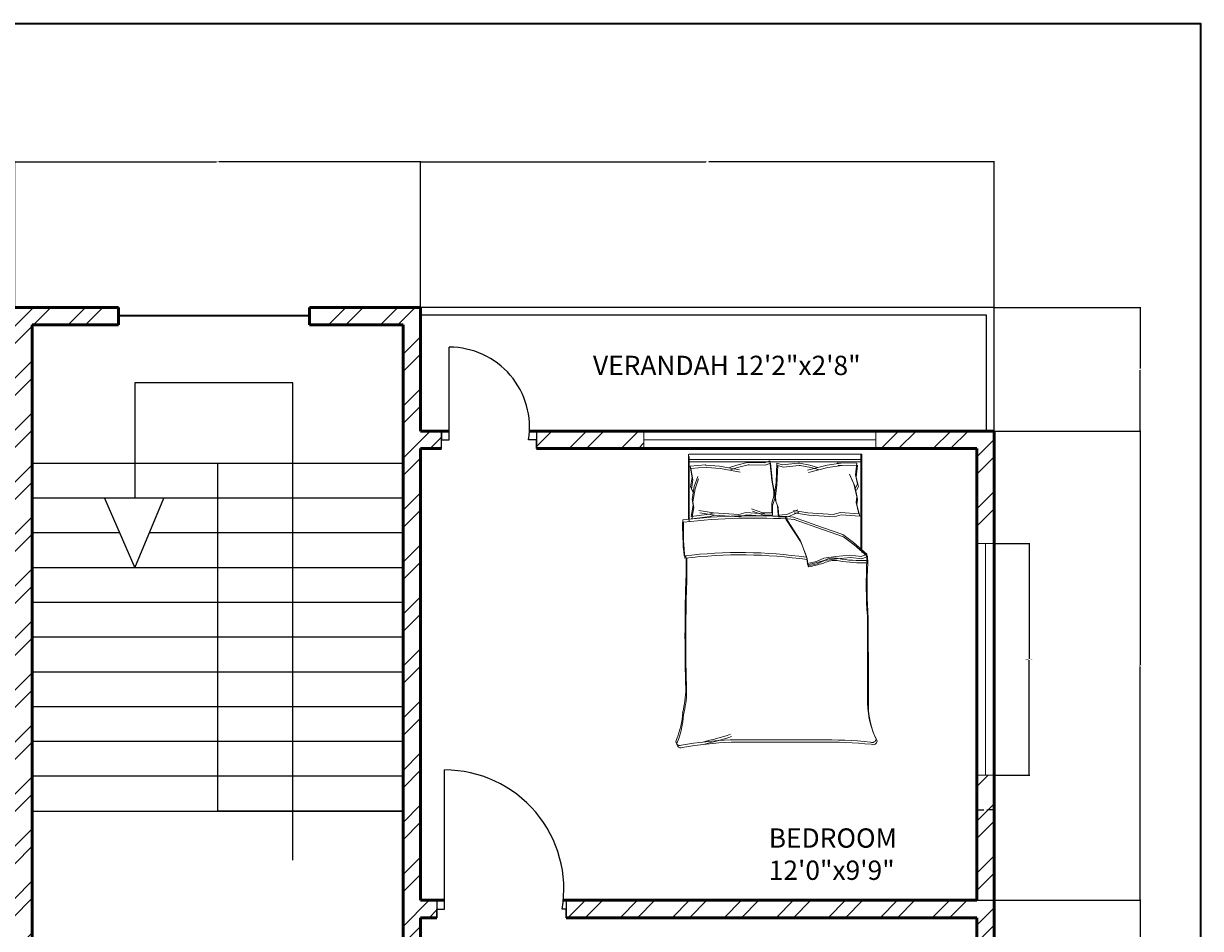
# Model space of a CAD drawing. Units: inches. Extents: x 2129 to 2642, y 1542 to 2414.
# Tile 9 of 9: x 2338 to 2642, y 2179 to 2414. Entities that reach past the tile are written whole.
import ezdxf

# ---------------------------------------------------------------- set-up
doc = ezdxf.new("R2010")
doc.units = ezdxf.units.IN
for name, color, linetype, lineweight in [('A-ANNO-DIMS', 2, 'Continuous', 18), ('A-ANNO-TTLB', 7, 'Continuous', 35), ('A-AREA-IDEN', 7, 'Continuous', 18), ('A-DOOR', 3, 'Continuous', 25), ('A-FLOR-RAIL', 80, 'Continuous', 25), ('A-FLOR-STRS', 11, 'Continuous', 25), ('A-FURN', 8, 'Continuous', 18), ('A-GLAZ', 4, 'Continuous', 18), ('A-WALL', 7, 'Continuous', 50), ('A-WALL-PATT', 252, 'Continuous', 13)]:
    doc.layers.add(name, color=color, linetype=linetype, lineweight=lineweight)
doc.styles.get("Standard").update_dxf_attribs({"font": 'arial.ttf'})
doc.dimstyles.get("Standard").update_dxf_attribs({"dimtxt": 0.18, "dimasz": 0.18, "dimexe": 0.18, "dimexo": 0.0625, "dimgap": 0.09, "dimtad": 0, "dimtih": 1, "dimtoh": 1, "dimdec": 4, "dimzin": 0, "dimdsep": 46, "dimtxsty": 'Standard', "dimcen": 0.09, "dimadec": 0, "dimazin": 0, "dimtfac": 1, "dimtdec": 4, "dimtofl": 0, "dimtmove": 0, "dimatfit": 3, "dimfxl": 1, "dimtolj": 1, "dimtzin": 0, "dimarcsym": 0})

# ---------------------------------------------------------------- blocks, each defined once
blk = doc.blocks.new('BED-DOUBLE')
for p, q in [((3.24, 59.14), (3.24, 76.05)), ((3.24, 74.61), (47.87, 74.61)), ((3.25, 59.14), (3.25, 76.05)), ((3.25, 74.61), (47.87, 74.61)), ((48.08, 76.05), (3.46, 76.05)), ((3.46, 58.54), (3.46, 75.45)), ((3.46, 58.54), (3.46, 75.45)), ((3.46, 74.02), (48.08, 74.02)), ((3.46, 74.02), (48.08, 74.02)), ((3.64, 72.93), (7.64, 73.24)), ((3.64, 72.93), (7.64, 73.24)), ((7.64, 73.24), (7.74, 73.22)), ((7.64, 73.24), (7.74, 73.22)), ((7.74, 73.22), (11.31, 72.95)), ((7.74, 73.22), (11.31, 72.95)), ((13.87, 72.55), (15.76, 73.22)), ((13.87, 72.55), (15.76, 73.22)), ((15.76, 73.22), (18.46, 73.9)), ((15.76, 73.22), (18.46, 73.9)), ((15.97, 72.62), (18.67, 73.3)), ((15.97, 72.62), (18.67, 73.3)), ((18.46, 73.9), (18.76, 73.9)), ((18.46, 73.9), (18.76, 73.9)), ((18.67, 73.3), (18.97, 73.3)), ((18.67, 73.3), (18.97, 73.3)), ((18.76, 73.9), (22.91, 73.76)), ((18.76, 73.9), (22.91, 73.76)), ((18.97, 73.3), (23.12, 73.16)), ((18.97, 73.3), (23.12, 73.16)), ((22.91, 73.76), (24.26, 74.3)), ((22.91, 73.76), (24.26, 74.3)), ((23.12, 73.16), (24.47, 73.7)), ((23.12, 73.16), (24.47, 73.7)), ((24.26, 74.3), (24.8, 69.31)), ((24.26, 74.3), (24.8, 69.31)), ((24.47, 73.7), (25.01, 68.71)), ((24.47, 73.7), (25.01, 68.71)), ((26.12, 73.72), (25.9, 68.7)), ((26.12, 73.72), (25.9, 68.7)), ((26.34, 73.12), (26.11, 68.1)), ((26.34, 73.12), (26.11, 68.1)), ((27.5, 73.27), (26.12, 73.72)), ((27.5, 73.27), (26.12, 73.72)), ((27.72, 72.67), (26.34, 73.12)), ((27.72, 72.67), (26.34, 73.12)), ((31.64, 73.66), (27.5, 73.27)), ((31.64, 73.66), (27.5, 73.27)), ((31.94, 73.68), (31.64, 73.66)), ((31.94, 73.68), (31.64, 73.66)), ((34.68, 73.17), (31.94, 73.68)), ((34.67, 73.17), (31.94, 73.68)), ((39.14, 73.18), (34.08, 71.92)), ((39.14, 73.18), (34.08, 71.92)), ((36.6, 72.62), (34.67, 73.17)), ((36.6, 72.62), (34.68, 73.17)), ((42.68, 73.67), (39.14, 73.18)), ((42.68, 73.67), (39.14, 73.18)), ((46.79, 73.66), (41.75, 73.75)), ((41.75, 73.75), (42.68, 73.67)), ((46.79, 73.66), (41.75, 73.75)), ((41.75, 73.75), (42.68, 73.67)), ((47.01, 73.06), (41.96, 73.15)), ((41.96, 73.15), (42.9, 73.08)), ((47.01, 73.06), (41.96, 73.15)), ((41.96, 73.15), (42.9, 73.08)), ((46.79, 73.66), (46.44, 70.66)), ((46.79, 73.66), (46.44, 70.66)), ((47.87, 76.05), (47.87, 51.2)), ((47.87, 76.05), (47.87, 51.2)), ((48.08, 76.05), (48.08, 75.45)), ((48.08, 75.45), (48.08, 50.6)), ((48.08, 75.45), (48.08, 50.6)), ((3.64, 72.95), (4.18, 69.98)), ((3.64, 72.95), (4.18, 69.98)), ((3.85, 72.33), (7.85, 72.64)), ((3.85, 72.33), (7.85, 72.64)), ((3.85, 72.35), (4.39, 69.38)), ((3.85, 72.35), (4.39, 69.38)), ((4.72, 67.69), (5.66, 70.25)), ((4.72, 67.69), (5.66, 70.25)), ((7.85, 72.64), (7.95, 72.62)), ((7.85, 72.64), (7.95, 72.62)), ((7.95, 72.62), (11.52, 72.35)), ((7.95, 72.62), (11.52, 72.35)), ((11.31, 72.95), (16.44, 72.01)), ((11.31, 72.95), (16.44, 72.01)), ((11.52, 72.35), (16.65, 71.41)), ((11.52, 72.35), (16.65, 71.41)), ((14.08, 71.95), (15.97, 72.62)), ((14.08, 71.95), (15.97, 72.62)), ((31.85, 73.06), (27.72, 72.67)), ((31.85, 73.06), (27.72, 72.67)), ((32.15, 73.08), (31.85, 73.06)), ((32.15, 73.08), (31.85, 73.06)), ((34.89, 72.58), (32.15, 73.08)), ((34.89, 72.58), (32.15, 73.08)), ((39.35, 72.58), (34.29, 71.32)), ((39.35, 72.58), (34.29, 71.32)), ((36.82, 72.02), (34.89, 72.58)), ((36.82, 72.02), (34.89, 72.58)), ((42.9, 73.08), (39.35, 72.58)), ((42.9, 73.08), (39.35, 72.58)), ((46.04, 68.34), (44.94, 70.84)), ((46.04, 68.34), (44.94, 70.84)), ((46.26, 67.74), (45.15, 70.24)), ((46.26, 67.74), (45.15, 70.24)), ((46.44, 70.66), (46.99, 68.26)), ((46.44, 70.66), (46.99, 68.26)), ((47.01, 73.06), (46.65, 70.06)), ((47.01, 73.06), (46.65, 70.06)), ((46.65, 70.06), (47.21, 67.66)), ((46.65, 70.06), (47.21, 67.66)), ((4.18, 69.98), (3.77, 67.55)), ((4.18, 69.98), (3.77, 67.55)), ((3.77, 67.55), (4.31, 66.61)), ((3.77, 67.55), (4.31, 66.61)), ((4.39, 69.38), (3.98, 66.95)), ((4.39, 69.38), (3.99, 66.95)), ((4.18, 64.31), (4.72, 67.69)), ((4.18, 64.31), (4.72, 67.69)), ((4.39, 63.71), (4.93, 67.09)), ((4.39, 63.71), (4.93, 67.09)), ((4.93, 67.09), (5.87, 69.65)), ((4.93, 67.09), (5.87, 69.65)), ((24.8, 69.31), (25.34, 66.34)), ((24.8, 69.31), (25.34, 66.34)), ((25.01, 68.71), (25.55, 65.74)), ((25.01, 68.71), (25.55, 65.74)), ((25.9, 68.7), (25.54, 65.7)), ((25.9, 68.7), (25.54, 65.7)), ((26.11, 68.1), (25.76, 65.11)), ((26.11, 68.1), (25.76, 65.11)), ((46.79, 65), (46.04, 68.34)), ((46.79, 65), (46.04, 68.34)), ((47.01, 64.41), (46.26, 67.74)), ((47.01, 64.41), (46.26, 67.74)), ((46.99, 68.26), (46.51, 67.28)), ((46.99, 68.26), (46.51, 67.28)), ((47.21, 67.66), (46.73, 66.69)), ((47.21, 67.66), (46.73, 66.69)), ((3.98, 66.95), (4.52, 66.01)), ((3.99, 66.95), (4.53, 66.01)), ((4.45, 62.82), (4.18, 64.31)), ((4.45, 62.82), (4.18, 64.31)), ((25.34, 65.12), (24.8, 63.36)), ((25.34, 65.12), (24.8, 63.36)), ((25.55, 64.52), (25.01, 62.77)), ((25.55, 64.52), (25.01, 62.77)), ((25.34, 66.34), (25.34, 65.12)), ((25.34, 66.34), (25.34, 65.12)), ((25.54, 65.7), (25.62, 64.49)), ((25.54, 65.7), (25.62, 64.49)), ((25.55, 65.74), (25.55, 64.52)), ((25.55, 65.74), (25.55, 64.52)), ((25.62, 64.49), (26.27, 62.77)), ((25.62, 64.49), (26.27, 62.77)), ((25.76, 65.11), (25.83, 63.89)), ((25.76, 65.11), (25.83, 63.89)), ((46.62, 63.5), (46.79, 65)), ((46.62, 63.5), (46.79, 65)), ((46.83, 62.91), (47.01, 64.41)), ((46.83, 62.91), (47.01, 64.41)), ((3.91, 59.85), (4.45, 62.82)), ((3.91, 59.85), (4.45, 62.82)), ((4.12, 59.26), (4.66, 62.23)), ((4.12, 59.26), (4.66, 62.23)), ((4.66, 62.23), (4.39, 63.71)), ((4.66, 62.23), (4.39, 63.71)), ((5.96, 61.45), (9.72, 60.83)), ((5.96, 61.45), (9.72, 60.83)), ((16.27, 60.43), (18.1, 60.95)), ((16.27, 60.43), (18.1, 60.95)), ((18.1, 60.95), (22.89, 60.57)), ((18.1, 60.95), (22.89, 60.57)), ((22.51, 60.86), (19.57, 61.88)), ((22.51, 60.86), (19.57, 61.88)), ((22.72, 60.26), (19.78, 61.28)), ((22.72, 60.26), (19.78, 61.28)), ((24.8, 63.36), (24.8, 60.86)), ((24.8, 63.36), (24.8, 60.86)), ((25.01, 62.77), (25.01, 60.26)), ((25.01, 62.77), (25.01, 60.26)), ((25.83, 63.89), (26.48, 62.18)), ((25.83, 63.89), (26.48, 62.18)), ((26.27, 62.77), (26.42, 60.27)), ((26.27, 62.77), (26.42, 60.27)), ((26.48, 62.18), (26.64, 59.68)), ((26.48, 62.18), (26.64, 59.68)), ((28.71, 60.42), (31.58, 61.62)), ((28.71, 60.42), (31.58, 61.62)), ((28.93, 59.82), (31.79, 61.02)), ((28.93, 59.82), (31.79, 61.02)), ((30.41, 61.45), (34.17, 60.83)), ((30.41, 61.45), (34.17, 60.83)), ((40.72, 60.43), (42.55, 60.95)), ((40.72, 60.43), (42.55, 60.95)), ((42.55, 60.95), (47.34, 60.57)), ((42.55, 60.95), (47.34, 60.57)), ((47.34, 60.57), (46.62, 63.5)), ((47.34, 60.57), (46.62, 63.5)), ((47.55, 59.98), (46.83, 62.91)), ((47.55, 59.98), (46.83, 62.91)), ((8.67, 60.53), (3.91, 59.85)), ((8.67, 60.53), (3.91, 59.85)), ((8.88, 59.93), (4.12, 59.26)), ((8.88, 59.93), (4.12, 59.26)), ((6.17, 60.86), (9.94, 60.23)), ((6.17, 60.86), (9.94, 60.23)), ((9.72, 60.83), (8.67, 60.53)), ((9.72, 60.83), (8.67, 60.53)), ((9.94, 60.23), (8.88, 59.93)), ((9.94, 60.23), (8.88, 59.93)), ((9.72, 60.83), (16.27, 60.43)), ((9.72, 60.83), (16.27, 60.43)), ((9.94, 60.23), (16.48, 59.83)), ((9.94, 60.23), (16.48, 59.83)), ((16.48, 59.83), (18.31, 60.35)), ((16.48, 59.83), (18.31, 60.35)), ((18.31, 60.35), (23.11, 59.98)), ((18.31, 60.35), (23.1, 59.98)), ((24.8, 60.86), (22.51, 60.86)), ((24.8, 60.86), (22.51, 60.86)), ((25.01, 60.26), (22.72, 60.26)), ((25.01, 60.26), (22.72, 60.26)), ((26.42, 60.27), (28.71, 60.42)), ((26.42, 60.27), (28.71, 60.42)), ((26.64, 59.68), (28.93, 59.82)), ((26.64, 59.68), (28.93, 59.82)), ((28.25, 59.82), (32.17, 53.75)), ((28.25, 59.82), (32.17, 53.75)), ((28.47, 59.22), (32.38, 53.16)), ((28.47, 59.22), (32.38, 53.16)), ((37.95, 57.08), (30.17, 59.82)), ((37.95, 57.08), (30.17, 59.82)), ((38.16, 56.48), (30.38, 59.22)), ((38.16, 56.48), (30.38, 59.22)), ((30.62, 60.86), (34.39, 60.23)), ((30.62, 60.86), (34.38, 60.23)), ((34.17, 60.83), (40.72, 60.43)), ((34.17, 60.83), (40.72, 60.43)), ((34.38, 60.23), (40.93, 59.83)), ((34.39, 60.23), (40.93, 59.83)), ((40.93, 59.83), (42.76, 60.35)), ((40.93, 59.83), (42.76, 60.35)), ((42.76, 60.35), (47.55, 59.98)), ((42.76, 60.35), (47.55, 59.98)), ((43.16, 55.2), (37.95, 57.08)), ((43.16, 55.2), (37.95, 57.08)), ((43.37, 54.6), (38.16, 56.48)), ((43.37, 54.6), (38.16, 56.48)), ((45.91, 53.17), (43.16, 55.2)), ((45.91, 53.17), (43.16, 55.2)), ((32.17, 53.75), (33.76, 49.56)), ((32.17, 53.75), (33.76, 49.56)), ((32.38, 53.16), (33.97, 48.96)), ((32.38, 53.16), (33.97, 48.96)), ((46.12, 52.58), (43.37, 54.6)), ((46.12, 52.58), (43.37, 54.6)), ((49.37, 50.14), (45.91, 53.17)), ((49.36, 50.14), (45.91, 53.17)), ((49.58, 49.54), (46.12, 52.58)), ((49.58, 49.54), (46.12, 52.58)), ((33.76, 49.56), (34.05, 47.68)), ((33.76, 49.56), (34.05, 47.68)), ((33.97, 48.96), (34.26, 47.09)), ((33.97, 48.96), (34.26, 47.09)), ((36.36, 48.26), (38.24, 49.13)), ((36.36, 48.26), (38.24, 49.13)), ((38.24, 49.13), (41.42, 49.56)), ((38.24, 49.13), (41.42, 49.56)), ((38.45, 48.53), (41.64, 48.96)), ((38.45, 48.53), (41.64, 48.96)), ((41.42, 49.56), (45.04, 49.85)), ((41.42, 49.56), (45.04, 49.85)), ((41.64, 48.96), (45.25, 49.25)), ((41.64, 48.96), (45.25, 49.25)), ((45.04, 49.85), (47.93, 49.56)), ((45.04, 49.85), (47.93, 49.56)), ((45.25, 49.25), (48.14, 48.96)), ((45.25, 49.25), (48.14, 48.96)), ((47.93, 49.56), (49.37, 50.14)), ((47.93, 49.56), (49.36, 50.14)), ((48.14, 48.96), (49.58, 49.54)), ((48.14, 48.96), (49.58, 49.54)), ((49.44, 48.51), (49.36, 50.14, 3.61)), ((49.44, 48.51), (49.37, 50.14, 3.61)), ((49.65, 47.91), (49.58, 49.54, 3.61)), ((49.65, 47.91), (49.58, 49.54, 3.61)), ((34.05, 47.68), (36.36, 48.26)), ((34.05, 47.68), (36.36, 48.26)), ((34.26, 47.09), (36.57, 47.66)), ((34.26, 47.09), (36.57, 47.66)), ((36.57, 47.66), (38.45, 48.53)), ((36.57, 47.66), (38.45, 48.53)), ((14.07, 2.05), (37.05, 2.05)), ((14.07, 2.05), (37.05, 2.05)), ((14.28, 1.46), (37.26, 1.46)), ((14.28, 1.46), (37.26, 1.46))]:
    blk.add_line(p, q)
for centre, radius, start, end in [((79.52, 57.28), 77.79, 178.7218, 185.604), ((79.52, 57.28), 77.79, 178.7218, 185.604), ((19.94, -93.94), 154.04, 86.0865, 96.7821), ((19.94, -93.94), 154.04, 86.0865, 96.7821), ((79.73, 56.69), 77.79, 178.7218, 185.604), ((79.73, 56.69), 77.79, 178.7218, 185.604), ((20.16, -94.54), 154.04, 86.0865, 96.7821), ((20.16, -94.54), 154.04, 86.0865, 96.7821), ((16.58, -69.91), 120.47, 81.7845, 96.9006), ((16.58, -69.91), 120.47, 81.7845, 96.9006), ((16.79, -70.51), 120.47, 81.7845, 96.9006), ((16.79, -70.51), 120.47, 81.7845, 96.9006), ((-156.22, 46.94), 158.84, 358.4762, 1.0082), ((-156.22, 46.94), 158.84, 358.4762, 1.0082), ((-156.01, 46.34), 158.84, 358.4762, 1.0082), ((-156.01, 46.34), 158.84, 358.4762, 1.0082), ((40.85, 43.3), 5.81, 78.6608, 113.7384), ((40.85, 43.3), 5.81, 78.6608, 113.7384), ((47.93, 82.26), 33.79, 259.8763, 272.5657), ((47.93, 82.26), 33.79, 259.8763, 272.5657), ((34.21, 47.62), 0.172, 160.2464, 271.1377), ((34.21, 47.62), 0.172, 160.2464, 271.1377), ((29.09, 74.66), 27.69, 280.6617, 289.8806), ((29.09, 74.66), 27.69, 280.6617, 289.8806), ((34.42, 47.03), 0.172, 160.2464, 271.1377), ((34.42, 47.03), 0.172, 160.2464, 271.1377), ((29.3, 74.07), 27.69, 280.6617, 289.8806), ((29.3, 74.07), 27.69, 280.6617, 289.8806), ((41.06, 42.71), 5.81, 78.6608, 113.7384), ((41.06, 42.71), 5.81, 78.6608, 113.7384), ((48.14, 81.67), 33.79, 259.8763, 272.5657), ((48.14, 81.67), 33.79, 259.8763, 272.5657), ((170.19, 42.14), 120.92, 176.9791, 183.8365), ((170.19, 42.14), 120.92, 176.9791, 183.8365), ((170.4, 41.54), 120.92, 176.9791, 183.8365), ((170.4, 41.54), 120.92, 176.9791, 183.8365), ((452.7, 28.79), 450.36, 178.2277, 181.7185), ((452.7, 28.79), 450.36, 178.2277, 181.7185), ((452.91, 28.19), 450.36, 178.2277, 181.7185), ((452.91, 28.19), 450.36, 178.2277, 181.7185), ((-4210.02, 12.72), 4259.62, 0.00217, 0.28689), ((-4210.02, 12.72), 4259.62, 0.00217, 0.28689), ((-4209.81, 12.12), 4259.62, 0.00217, 0.28689), ((-4209.81, 12.12), 4259.62, 0.00217, 0.28689), ((-25.12, 15.81), 27.67, 346.0648, 358.9113), ((-25.12, 15.81), 27.67, 346.0648, 358.9113), ((-24.9, 15.21), 27.67, 346.0648, 358.9113), ((-24.9, 15.21), 27.67, 346.0648, 358.9113), ((71.11, 11.93), 21.54, 177.4714, 206.4681), ((71.11, 11.93), 21.54, 177.4714, 206.4681), ((71.33, 11.33), 21.54, 177.4714, 206.4681), ((71.32, 11.33), 21.54, 177.4714, 206.4681), ((-20.22, 10.43), 22, 337.9751, 356.652), ((-20.22, 10.43), 22, 337.9751, 356.652), ((-20.01, 9.83), 22, 337.9751, 356.652), ((-20.01, 9.83), 22, 337.9751, 356.652), ((-16.08, 98.19), 99.41, 283.3832, 287.7053), ((-16.08, 98.19), 99.41, 283.3832, 287.7053), ((1.02, 1.61), 1.02, 146.1736, 293.4781), ((1.02, 1.61), 1.02, 146.1736, 293.4781), ((1.23, 1.01), 1.02, 146.1736, 293.4781), ((1.23, 1.01), 1.02, 146.1736, 293.4781), ((20.01, -111.48), 113.69, 92.9958, 99.4091), ((20.01, -111.48), 113.69, 92.9958, 99.4091), ((20.22, -112.08), 113.69, 92.9958, 99.4091), ((20.22, -112.08), 113.69, 92.9958, 99.4091), ((-15.87, 97.59), 99.41, 283.3832, 287.7053), ((-15.87, 97.59), 99.41, 283.3832, 287.7053), ((38.43, -122.17), 124.23, 84.4998, 90.6351), ((38.43, -122.17), 124.23, 84.4998, 90.6351), ((38.64, -122.76), 124.23, 84.4998, 90.6351), ((38.64, -122.76), 124.23, 84.4998, 90.6351), ((50.81, 2.4), 1.03, 242.6588, 356.02), ((50.81, 2.4), 1.03, 242.6588, 356.02), ((51.02, 1.81), 1.03, 242.6588, 356.02), ((51.02, 1.81), 1.03, 242.6588, 356.02)]:
    blk.add_arc(centre, radius, start, end)
blk = doc.blocks.new('WIN-60-A')
for p, q in [((0, 4.5), (0, 0)), ((60, 2.25), (60, 4.5)), ((60, 4.5), (60, 0)), ((0, 0), (0, 2.25)), ((0, 2.25), (60, 2.25))]:
    blk.add_line(p, q)
blk = doc.blocks.new('WIN-60-B')
for p, q in [((4.5, 60), (0, 60)), ((0, 60), (2.25, 60)), ((2.25, 60), (2.25, 0)), ((2.25, 0), (0, 0)), ((0, 0), (4.5, 0))]:
    blk.add_line(p, q)
blk = doc.blocks.new('*D16')
at = {"layer": 'A-ANNO-DIMS', "color": 0, "lineweight": -2, "transparency": 16777216}
for p, q in [((2588.97, 2279.11), (2598.08, 2279.11)), ((2597.9, 2278.93), (2597.9, 2249.29)), ((2597.9, 2219.29), (2597.9, 2248.93)), ((2588.97, 2219.11), (2598.08, 2219.11))]:
    blk.add_line(p, q, dxfattribs=at)
at = {"layer": 'A-ANNO-DIMS', "color": 0, "transparency": 16777216}
for points in [[(2597.87, 2278.93), (2597.93, 2278.93), (2597.9, 2279.11)], [(2597.87, 2219.29), (2597.93, 2219.29), (2597.9, 2219.11)]]:
    blk.add_solid(points, dxfattribs=at)
at = {"layer": 'Defpoints', "color": 0, "transparency": 16777216}
for p in [(2588.9, 2279.11), (2588.9, 2219.11), (2597.9, 2219.11)]:
    blk.add_point(p, dxfattribs=at)
at = {"layer": 'A-ANNO-DIMS', "color": 0, "transparency": 16777216, "insert": (2597.9, 2249.11), "char_height": 0.18, "attachment_point": 5}
blk.add_mtext('\\A1;WINDOW B 60 TYP.', dxfattribs=at)
blk = doc.blocks.new('*D17')
at = {"layer": 'A-ANNO-DIMS', "color": 0, "lineweight": -2, "transparency": 16777216}
for p, q in [((2584.4, 2219.05), (2584.4, 2209.93)), ((2588.9, 2219.05), (2588.9, 2209.93)), ((2584.58, 2210.11), (2586.2, 2210.11)), ((2588.72, 2210.11), (2587.11, 2210.11))]:
    blk.add_line(p, q, dxfattribs=at)
at = {"layer": 'A-ANNO-DIMS', "color": 0, "transparency": 16777216}
for points in [[(2584.58, 2210.14), (2584.58, 2210.08), (2584.4, 2210.11)], [(2588.72, 2210.14), (2588.72, 2210.08), (2588.9, 2210.11)]]:
    blk.add_solid(points, dxfattribs=at)
at = {"layer": 'Defpoints', "color": 0, "transparency": 16777216}
for p in [(2584.4, 2219.11), (2588.9, 2219.11), (2584.4, 2210.11)]:
    blk.add_point(p, dxfattribs=at)
at = {"layer": 'A-ANNO-DIMS', "color": 0, "transparency": 16777216, "insert": (2586.65, 2210.11), "char_height": 0.18, "attachment_point": 5}
blk.add_mtext('\\A1;5 TYP.', dxfattribs=at)
blk = doc.blocks.new('*D37')
at = {"layer": 'A-ANNO-DIMS', "color": 0, "lineweight": -2, "transparency": 16777216}
for p, q in [((2335.4, 2340.28), (2335.4, 2378.15)), ((2335.58, 2377.97), (2387.62, 2377.97)), ((2440.22, 2377.97), (2388.19, 2377.97)), ((2440.4, 2340.28), (2440.4, 2378.15))]:
    blk.add_line(p, q, dxfattribs=at)
at = {"layer": 'A-ANNO-DIMS', "color": 0, "transparency": 16777216}
for points in [[(2335.58, 2378), (2335.58, 2377.94), (2335.4, 2377.97)], [(2440.22, 2378), (2440.22, 2377.94), (2440.4, 2377.97)]]:
    blk.add_solid(points, dxfattribs=at)
at = {"layer": 'Defpoints', "color": 0, "transparency": 16777216}
for p in [(2440.4, 2377.97), (2335.4, 2340.22), (2440.4, 2340.22)]:
    blk.add_point(p, dxfattribs=at)
at = {"layer": 'A-ANNO-DIMS', "color": 0, "transparency": 16777216, "insert": (2387.9, 2377.97), "char_height": 0.18, "attachment_point": 5}
blk.add_mtext('\\A1;105', dxfattribs=at)
blk = doc.blocks.new('*D38')
at = {"layer": 'A-ANNO-DIMS', "color": 0, "lineweight": -2, "transparency": 16777216}
for p, q in [((2440.4, 2340.28), (2440.4, 2378.15)), ((2440.58, 2377.97), (2514.27, 2377.97)), ((2588.72, 2377.97), (2515.04, 2377.97)), ((2588.9, 2340.28), (2588.9, 2378.15))]:
    blk.add_line(p, q, dxfattribs=at)
at = {"layer": 'A-ANNO-DIMS', "color": 0, "transparency": 16777216}
for points in [[(2440.58, 2378), (2440.58, 2377.94), (2440.4, 2377.97)], [(2588.72, 2378), (2588.72, 2377.94), (2588.9, 2377.97)]]:
    blk.add_solid(points, dxfattribs=at)
at = {"layer": 'Defpoints', "color": 0, "transparency": 16777216}
for p in [(2588.9, 2377.97), (2440.4, 2340.22), (2588.9, 2340.22)]:
    blk.add_point(p, dxfattribs=at)
at = {"layer": 'A-ANNO-DIMS', "color": 0, "transparency": 16777216, "insert": (2514.65, 2377.97), "char_height": 0.18, "attachment_point": 5}
blk.add_mtext('\\A1;148.5', dxfattribs=at)
blk = doc.blocks.new('*D44')
at = {"layer": 'A-ANNO-DIMS', "color": 0, "lineweight": -2, "transparency": 16777216}
for p, q in [((2584.47, 2186.72), (2626.83, 2186.72)), ((2626.65, 2186.54), (2626.65, 2125.65)), ((2626.65, 2064.4), (2626.65, 2125.29)), ((2584.47, 2064.22), (2626.83, 2064.22))]:
    blk.add_line(p, q, dxfattribs=at)
at = {"layer": 'A-ANNO-DIMS', "color": 0, "transparency": 16777216}
for points in [[(2626.62, 2186.54), (2626.68, 2186.54), (2626.65, 2186.72)], [(2626.62, 2064.4), (2626.68, 2064.4), (2626.65, 2064.22)]]:
    blk.add_solid(points, dxfattribs=at)
at = {"layer": 'Defpoints', "color": 0, "transparency": 16777216}
for p in [(2584.4, 2186.72), (2626.65, 2186.72), (2584.4, 2064.22)]:
    blk.add_point(p, dxfattribs=at)
at = {"layer": 'A-ANNO-DIMS', "color": 0, "transparency": 16777216, "insert": (2626.65, 2125.47), "char_height": 0.18, "attachment_point": 5}
blk.add_mtext('\\A1;122.5', dxfattribs=at)
blk = doc.blocks.new('*D45')
at = {"layer": 'A-ANNO-DIMS', "color": 0, "lineweight": -2, "transparency": 16777216}
for p, q in [((2588.97, 2308.22), (2626.83, 2308.22)), ((2626.65, 2308.04), (2626.65, 2247.65)), ((2626.65, 2186.9), (2626.65, 2247.29)), ((2584.47, 2186.72), (2626.83, 2186.72))]:
    blk.add_line(p, q, dxfattribs=at)
at = {"layer": 'A-ANNO-DIMS', "color": 0, "transparency": 16777216}
for points in [[(2626.62, 2308.04), (2626.68, 2308.04), (2626.65, 2308.22)], [(2626.62, 2186.9), (2626.68, 2186.9), (2626.65, 2186.72)]]:
    blk.add_solid(points, dxfattribs=at)
at = {"layer": 'Defpoints', "color": 0, "transparency": 16777216}
for p in [(2588.9, 2308.22), (2626.65, 2308.22), (2584.4, 2186.72)]:
    blk.add_point(p, dxfattribs=at)
at = {"layer": 'A-ANNO-DIMS', "color": 0, "transparency": 16777216, "insert": (2626.65, 2247.47), "char_height": 0.18, "attachment_point": 5}
blk.add_mtext('\\A1;121.5', dxfattribs=at)
blk = doc.blocks.new('*D46')
at = {"layer": 'A-ANNO-DIMS', "color": 0, "lineweight": -2, "transparency": 16777216}
for p, q in [((2588.97, 2340.22), (2626.83, 2340.22)), ((2626.65, 2340.04), (2626.65, 2324.4)), ((2626.65, 2308.4), (2626.65, 2324.04)), ((2588.97, 2308.22), (2626.83, 2308.22))]:
    blk.add_line(p, q, dxfattribs=at)
at = {"layer": 'A-ANNO-DIMS', "color": 0, "transparency": 16777216}
for points in [[(2626.62, 2340.04), (2626.68, 2340.04), (2626.65, 2340.22)], [(2626.62, 2308.4), (2626.68, 2308.4), (2626.65, 2308.22)]]:
    blk.add_solid(points, dxfattribs=at)
at = {"layer": 'Defpoints', "color": 0, "transparency": 16777216}
for p in [(2588.9, 2340.22), (2626.65, 2340.22), (2588.9, 2308.22)]:
    blk.add_point(p, dxfattribs=at)
at = {"layer": 'A-ANNO-DIMS', "color": 0, "transparency": 16777216, "insert": (2626.65, 2324.22), "char_height": 0.18, "attachment_point": 5}
blk.add_mtext('\\A1;32', dxfattribs=at)

msp = doc.modelspace()

# ---------------------------------------------------------------- hatches: boundary and pattern name
at = {"layer": 'A-WALL-PATT'}
h = msp.add_hatch(dxfattribs=at)
h.set_pattern_fill('ANSI32', color=256)
h.paths.add_polyline_path([(2306.2606, 2305.9717), (2306.2606, 2308.2217), (2276.3515, 2308.2217), (2276.3515, 2303.7217), (2306.2606, 2303.7217)])
h.paths.add_polyline_path([(2216.3515, 2305.9717), (2216.3515, 2308.2217), (2186.9043, 2308.2217), (2186.9043, 2278.1696), (2191.4043, 2278.1696), (2191.4043, 2303.7217), (2216.3515, 2303.7217)])
h.paths.add_polyline_path([(2339.9043, 2335.7217), (2362.1938, 2335.7217), (2362.1938, 2340.2217), (2335.4043, 2340.2217), (2335.4043, 2308.2217), (2329.3487, 2308.2217), (2329.3487, 2305.9717), (2329.3487, 2303.7217), (2335.4043, 2303.7217), (2335.4043, 2186.7217), (2329.4345, 2186.7217), (2329.4345, 2182.2217), (2335.4043, 2182.2217), (2335.4043, 2174.7178), (2339.9043, 2174.7178), (2339.9043, 2182.2217), (2339.9043, 2303.7217)])
h.paths.add_polyline_path([(2440.4043, 2340.2217), (2411.654, 2340.2217), (2411.654, 2335.7217), (2435.9043, 2335.7217), (2435.9043, 2303.7217), (2435.9043, 2182.2217), (2435.9043, 2174.1935), (2438.1543, 2174.1935), (2440.4043, 2174.1935), (2440.4043, 2182.2217), (2444.653, 2182.2217), (2444.653, 2184.4717), (2444.653, 2186.7217), (2440.4043, 2186.7217), (2440.4043, 2303.7217), (2445.8547, 2303.7217), (2445.8547, 2308.2217), (2440.4043, 2308.2217)])
h.paths.add_polyline_path([(2498.2381, 2308.2217), (2470.3901, 2308.2217), (2470.3901, 2303.7217), (2498.2381, 2303.7217), (2498.2381, 2305.9717)])
h.paths.add_polyline_path([(2588.9043, 2308.2217), (2586.9043, 2308.2217), (2558.2381, 2308.2217), (2558.2381, 2303.7217), (2584.4043, 2303.7217), (2584.4043, 2279.1087), (2588.9043, 2279.1087)])
h.paths.add_polyline_path([(2588.9043, 2219.1087), (2584.4043, 2219.1087), (2584.4043, 2186.7217), (2478.0667, 2186.7217), (2478.0667, 2182.2217), (2584.4043, 2182.2217), (2584.4043, 2157.7883), (2588.9043, 2157.7883)])
h.paths.add_polyline_path([(2588.9043, 2097.7883), (2584.6063, 2097.7883), (2584.6063, 2075.5462, -0.09241561), (2584.4043, 2074.4627), (2584.4043, 2064.2217), (2495.9043, 2064.2217), (2495.9043, 2040.4611), (2500.4043, 2040.4611), (2500.4043, 2059.7217), (2584.4043, 2059.7217), (2584.4043, 2052.2164), (2588.9043, 2052.2164)])
h.paths.add_polyline_path([(2588.9043, 2028.2164), (2584.4043, 2028.2164), (2584.4043, 2011.7217), (2500.4043, 2011.7217), (2500.4043, 2015.243), (2498.1543, 2015.243), (2495.9043, 2015.243), (2495.9043, 2007.2217), (2495.9043, 2003.7597), (2500.4043, 2003.7597), (2500.4043, 2007.2217), (2584.4043, 2007.2217), (2584.4043, 1992.1997), (2588.9043, 1992.1997)])
h.paths.add_polyline_path([(2588.9043, 1956.1997), (2584.4043, 1956.1997), (2584.4043, 1941.2217), (2500.4043, 1941.2217), (2500.4043, 1985.1493), (2498.1543, 1985.1493), (2495.9043, 1985.1493), (2495.9043, 1941.2217), (2435.9043, 1941.2217), (2435.9043, 1930.3963), (2440.4043, 1930.3963), (2440.4043, 1936.7217), (2584.4043, 1936.7217), (2584.4043, 1909.8406), (2588.9043, 1909.8406)])
h.paths.add_polyline_path([(2588.9043, 1849.8406), (2584.4043, 1849.8406), (2584.4043, 1801.3526), (2588.9043, 1801.3526)])
h.paths.add_polyline_path([(2584.4043, 1828.7217), (2495.9043, 1828.7217), (2440.4043, 1828.7217), (2440.4043, 1905.2159), (2438.1543, 1905.2159), (2435.9043, 1905.2159), (2435.9043, 1828.7217), (2428.9101, 1828.7217), (2428.9101, 1824.2217), (2584.4043, 1824.2217)])
h.paths.add_polyline_path([(2588.9043, 1741.3526), (2584.4043, 1741.3526), (2584.4043, 1704.2217), (2468.3173, 1704.2217), (2468.3173, 1701.9717), (2468.3173, 1699.7217), (2588.9043, 1699.7217)])
h.paths.add_polyline_path([(2442.4043, 1761.7217), (2435.0216, 1761.7217), (2435.0216, 1757.2217), (2437.9043, 1757.2217), (2437.9043, 1665.7217), (2442.4043, 1665.7217), (2442.4043, 1667.7217), (2442.4043, 1699.7217), (2446.6907, 1699.7217), (2446.6907, 1701.9717), (2446.6907, 1704.2217), (2442.4043, 1704.2217)])
h.paths.add_polyline_path([(2390.4043, 1757.2217), (2410.8996, 1757.2217), (2410.8996, 1761.7217), (2360.1741, 1761.7217), (2360.1741, 1759.4717), (2360.1741, 1757.2217), (2385.9043, 1757.2217), (2385.9043, 1674.8326), (2390.4043, 1674.8326)])
h.paths.add_polyline_path([(2337.9043, 1757.2217), (2340.3592, 1757.2217), (2340.3592, 1759.4717), (2340.3592, 1761.7217), (2333.4043, 1761.7217), (2333.4043, 1704.2217), (2327.381, 1704.2217), (2327.381, 1701.9717), (2327.381, 1699.7217), (2333.4043, 1699.7217), (2333.4043, 1665.7217), (2337.9043, 1665.7217)])
h.paths.add_polyline_path([(2191.4043, 1743.4804), (2186.9043, 1743.4804), (2186.9043, 1699.7217), (2188.9043, 1699.7217), (2191.4043, 1699.7217), (2306.5617, 1699.7217), (2306.5617, 1704.2217), (2191.4043, 1704.2217)])
h.paths.add_polyline_path([(2191.4043, 1859.8992), (2186.9043, 1859.8992), (2186.9043, 1803.4804), (2189.1543, 1803.4804), (2191.4043, 1803.4804)])
h.paths.add_polyline_path([(2352.5445, 1828.7217), (2191.4043, 1828.7217), (2191.4043, 1824.2217), (2333.4043, 1824.2217), (2352.5445, 1824.2217), (2352.5445, 1826.4717)])
h.paths.add_polyline_path([(2390.4043, 2085.328), (2385.9043, 2085.328), (2385.9043, 1828.7217), (2381.9668, 1828.7217), (2381.9668, 1826.4717), (2381.9668, 1824.2217), (2385.9043, 1824.2217), (2385.9043, 1761.7217), (2390.4043, 1761.7217), (2390.4043, 1824.2217), (2394.1868, 1824.2217), (2394.1868, 1827.6339), (2394.1868, 1828.7217), (2390.4043, 1828.7217)])
h.paths.add_polyline_path([(2339.9043, 1941.2217), (2335.4043, 1941.2217), (2279.9043, 1941.2217), (2279.9043, 1981.3432), (2277.6543, 1981.3432), (2275.4043, 1981.3432), (2275.4043, 1941.2217), (2191.4043, 1941.2217), (2191.4043, 1958.1079), (2186.9043, 1958.1079), (2186.9043, 1919.8992), (2189.1543, 1919.8992), (2191.4043, 1919.8992), (2191.4043, 1936.7217), (2279.9043, 1936.7217), (2335.4043, 1936.7217), (2335.4043, 1931.1382), (2339.9043, 1931.1382)])
h.paths.add_polyline_path([(2339.9043, 1902.7544), (2337.6543, 1902.7544), (2335.4043, 1902.7544), (2335.4043, 1828.7217), (2339.9043, 1828.7217)])
h.paths.add_polyline_path([(2279.9043, 2015.263), (2277.6543, 2015.263), (2275.4043, 2015.263), (2275.4043, 2011.7217), (2191.4043, 2011.7217), (2191.4043, 2026.6781), (2186.9043, 2026.6781), (2186.9043, 1994.1079), (2189.1543, 1994.1079), (2191.4043, 1994.1079), (2191.4043, 2007.2217), (2275.4043, 2007.2217), (2275.4043, 2003.2288), (2279.9043, 2003.2288), (2279.9043, 2007.2217)])
h.paths.add_polyline_path([(2296.0216, 2186.7217), (2191.4043, 2186.7217), (2191.4043, 2218.1696), (2186.9043, 2218.1696), (2186.9043, 2158.4509), (2191.4043, 2158.4509), (2191.4043, 2182.2217), (2296.0216, 2182.2217), (2296.0216, 2184.4717)])
h.paths.add_polyline_path([(2191.4043, 2098.4509), (2189.1543, 2098.4509), (2186.9043, 2098.4509), (2186.9043, 2050.6781), (2189.0487, 2050.6781), (2191.4043, 2050.6781), (2191.4043, 2059.7217), (2275.4043, 2059.7217), (2275.4043, 2038.4133), (2279.9043, 2038.4133), (2279.9043, 2064.2217), (2191.4043, 2064.2217)])
h.paths.add_polyline_path([(2268.3923, 1605.9386), (2516.3159, 1605.9386), (2516.3159, 1643.0314), (2268.3923, 1643.0314)], flags=9)
h.paths.add_polyline_path([(2399.6079, 1710.4489), (2428.8405, 1710.4489), (2428.8405, 1729.1062), (2399.6079, 1729.1062)], flags=9)
h.paths.add_polyline_path([(2342.1483, 1708.9956), (2371.3809, 1708.9956), (2371.3809, 1727.653), (2342.1483, 1727.653)], flags=9)
h.paths.add_polyline_path([(2200.7404, 1677.2519), (2282.3059, 1677.2519), (2282.3059, 1687.5555), (2200.7404, 1687.5555)], flags=9)
h.paths.add_polyline_path([(2209.8153, 1704.7448), (2250.627, 1704.7448), (2250.627, 1723.4021), (2209.8153, 1723.4021)], flags=25)
h.paths.add_polyline_path([(2213.9996, 1911.284), (2252.84, 1911.284), (2252.84, 1929.9413), (2213.9996, 1929.9413)], flags=9)
h.paths.add_polyline_path([(2210.8865, 1962.0987), (2244.0447, 1962.0987), (2244.0447, 1980.7561), (2210.8865, 1980.7561)], flags=25)
h.paths.add_polyline_path([(2219.0745, 2037.6131), (2248.2321, 2037.6131), (2248.2321, 2056.2705), (2219.0745, 2056.2705)], flags=9)
h.paths.add_polyline_path([(2379.9702, 2099.0686), (2409.3767, 2099.0686), (2409.3767, 2117.7259), (2379.9702, 2117.7259)], flags=9)
h.paths.add_polyline_path([(2375.9312, 2160.3752), (2405.3173, 2160.3752), (2405.3173, 2179.0325), (2375.9312, 2179.0325)], flags=9)
h.paths.add_polyline_path([(2269.5058, 2112.1824), (2310.3175, 2112.1824), (2310.3175, 2130.8397), (2269.5058, 2130.8397)], flags=9)
h.paths.add_polyline_path([(2209.6567, 2193.667), (2248.4971, 2193.667), (2248.4971, 2212.3243), (2209.6567, 2212.3243)], flags=25)
h.paths.add_polyline_path([(2491.6289, 1675.447), (2573.1944, 1675.447), (2573.1944, 1685.7506), (2491.6289, 1685.7506)], flags=9)
h.paths.add_polyline_path([(2492.0585, 1710.4489), (2530.8989, 1710.4489), (2530.8989, 1729.1062), (2492.0585, 1729.1062)], flags=25)
h.paths.add_polyline_path([(2495.6634, 1908.8646), (2534.5038, 1908.8646), (2534.5038, 1927.522), (2495.6634, 1927.522)], flags=9)
h.paths.add_polyline_path([(2516.7779, 1955.9942), (2549.9362, 1955.9942), (2549.9362, 1974.6516), (2516.7779, 1974.6516)], flags=25)
h.paths.add_polyline_path([(2509.7444, 2034.6896), (2538.902, 2034.6896), (2538.902, 2053.347), (2509.7444, 2053.347)], flags=9)
h.paths.add_polyline_path([(2467.8454, 2111.9593), (2508.6571, 2111.9593), (2508.6571, 2130.6167), (2467.8454, 2130.6167)], flags=9)
h.paths.add_polyline_path([(2528.5267, 2189.1742), (2567.3671, 2189.1742), (2567.3671, 2207.8316), (2528.5267, 2207.8316)], flags=25)
h.paths.add_polyline_path([(2483.7603, 2319.9841), (2557.5563, 2319.9841), (2557.5563, 2330.2877), (2483.7603, 2330.2877)], flags=9)
h.paths.add_polyline_path([(2204.078, 2317.0445), (2277.874, 2317.0445), (2277.874, 2327.3481), (2204.078, 2327.3481)], flags=9)

# ---------------------------------------------------------------- linework, layer by layer
at = {"layer": 'A-ANNO-TTLB'}
msp.add_lwpolyline([(2129.4387, 2413.7704), (2642.2731, 2413.7704), (2642.2731, 1542.3836), (2129.4387, 1542.3836)], close=True, dxfattribs=at)
at = {"layer": 'A-DOOR'}
for p, q in [((2447.8547, 2305.9717), (2447.8547, 2329.9717)), ((2445.8547, 2303.7217), (2445.8547, 2308.2217)), ((2445.8547, 2308.2217), (2445.8547, 2305.9717)), ((2445.8547, 2305.9717), (2447.8547, 2305.9717)), ((2470.3901, 2305.9717), (2468.3901, 2305.9717)), ((2470.3901, 2308.2217), (2470.3901, 2303.7217)), ((2470.3901, 2303.7217), (2470.3901, 2305.9717)), ((2446.653, 2184.4717), (2446.653, 2220.4717)), ((2444.653, 2186.7217), (2444.653, 2182.2217)), ((2444.653, 2182.2217), (2444.653, 2184.4717)), ((2444.653, 2184.4717), (2446.653, 2184.4717)), ((2478.0667, 2184.4717), (2477.0667, 2184.4717)), ((2478.0667, 2186.7217), (2478.0667, 2182.2217)), ((2478.0667, 2182.2217), (2478.0667, 2184.4717))]:
    msp.add_line(p, q, dxfattribs=at)
for centre, radius, start in [((2447.8547, 2309.1862), 20.7854, 351.103271), ((2446.653, 2189.6246), 30.8471, 350.383813)]:
    msp.add_arc(centre, radius, start, 90, dxfattribs=at)
at = {"layer": 'A-FLOR-RAIL'}
for p, q in [((2588.9043, 2340.2217), (2440.4043, 2340.2217)), ((2588.9043, 2308.2217), (2588.9043, 2340.2217)), ((2586.9043, 2338.2217), (2440.4043, 2338.2217)), ((2586.9043, 2308.2217), (2586.9043, 2338.2217))]:
    msp.add_line(p, q, dxfattribs=at)
at = {"layer": 'A-FLOR-STRS'}
for p, q in [((2407.3454, 2320.7067), (2366.4201, 2320.7067)), ((2366.4201, 2320.7067), (2366.4201, 2320.7067)), ((2366.4201, 2320.7067), (2366.4201, 2290.8397)), ((2407.3454, 2197.1032), (2407.3454, 2320.7067)), ((2435.9043, 2299.8397), (2339.9043, 2299.8397)), ((2387.9043, 2284.2403), (2387.9043, 2299.8397)), ((2435.9043, 2290.8397), (2339.9043, 2290.8397)), ((2358.6301, 2290.8397), (2366.4201, 2272.8397)), ((2373.9337, 2290.8397), (2360.9388, 2290.8397)), ((2366.4201, 2272.8397), (2373.9337, 2290.8397)), ((2362.5251, 2281.8397), (2339.9043, 2281.8397)), ((2435.9043, 2281.8397), (2370.1769, 2281.8397)), ((2387.9043, 2209.8397), (2387.9043, 2284.2403)), ((2435.9043, 2272.8397), (2339.9043, 2272.8397)), ((2435.9043, 2263.8397), (2339.9043, 2263.8397)), ((2435.9043, 2254.8397), (2339.9043, 2254.8397)), ((2435.9043, 2245.8397), (2339.9043, 2245.8397)), ((2435.9043, 2236.8397), (2339.9043, 2236.8397)), ((2435.9043, 2227.8397), (2339.9043, 2227.8397)), ((2435.9043, 2218.8397), (2339.9043, 2218.8397)), ((2339.9043, 2209.8397), (2435.9043, 2209.8397)), ((2435.9043, 2209.8397), (2387.9043, 2209.8397))]:
    msp.add_line(p, q, dxfattribs=at)
at = {"layer": 'A-GLAZ'}
for p, q in [((2411.654, 2338.2257), (2362.1938, 2338.2257)), ((2362.1938, 2337.9717), (2411.654, 2337.9717)), ((2411.654, 2337.9717), (2411.654, 2338.2257)), ((2411.654, 2337.9717), (2411.654, 2337.9717))]:
    msp.add_line(p, q, dxfattribs=at)
at = {"layer": 'A-WALL'}
for p, q in [((2335.4043, 2340.2217), (2362.1938, 2340.2217)), ((2362.1938, 2335.7217), (2362.1938, 2340.2217)), ((2411.654, 2335.7217), (2411.654, 2340.2217)), ((2411.654, 2340.2217), (2440.4043, 2340.2217)), ((2440.4043, 2308.2217), (2440.4043, 2340.2217)), ((2440.4043, 2340.2217), (2440.4043, 2335.7217)), ((2440.4043, 2340.2217), (2440.4043, 2338.2217)), ((2339.9043, 2303.7217), (2339.9043, 2335.7217)), ((2362.1938, 2335.7217), (2339.9043, 2335.7217)), ((2435.9043, 2335.7217), (2411.654, 2335.7217)), ((2435.9043, 2303.7217), (2435.9043, 2335.7217)), ((2440.4043, 2308.2217), (2447.8547, 2308.2217)), ((2440.4043, 2308.2217), (2447.8547, 2308.2217)), ((2468.6178, 2308.2217), (2588.9043, 2308.2217)), ((2468.6178, 2308.2217), (2588.9043, 2308.2217)), ((2588.9043, 2308.2217), (2588.9043, 1699.7217)), ((2339.9043, 2303.7217), (2339.9043, 2182.2217)), ((2435.9043, 2303.7217), (2435.9043, 2182.2217)), ((2440.4043, 2303.7217), (2440.4043, 2186.7217)), ((2440.4043, 2303.7217), (2445.8547, 2303.7217)), ((2470.3901, 2303.7217), (2584.4043, 2303.7217)), ((2584.4043, 2303.7217), (2584.4043, 2186.7217)), ((2440.4043, 2186.7217), (2446.653, 2186.7217)), ((2477.3632, 2186.7217), (2584.4043, 2186.7217)), ((2339.9043, 2182.2217), (2339.9043, 2174.7178)), ((2435.9043, 2182.2217), (2435.9043, 2174.1935)), ((2440.4043, 2182.2217), (2440.4043, 2172.9064)), ((2440.4043, 2182.2217), (2444.653, 2182.2217)), ((2478.0667, 2182.2217), (2584.4043, 2182.2217)), ((2584.4043, 2182.2217), (2584.4043, 2064.2217))]:
    msp.add_line(p, q, dxfattribs=at)

# ---------------------------------------------------------------- block references
at = {"layer": 'A-FURN'}
msp.add_blockref('BED-DOUBLE', (2506.5175, 2226.222), dxfattribs=at)
at = {"layer": 'A-GLAZ'}
msp.add_blockref('WIN-60-A', (2498.2385, 2303.722), dxfattribs=at)
at = {"layer": 'A-GLAZ', "rotation": 180}
msp.add_blockref('WIN-60-B', (2588.9047, 2279.1091), dxfattribs=at)

# ---------------------------------------------------------------- texts
at = {"layer": 'A-AREA-IDEN', "char_height": 5, "attachment_point": 1}
for s, width, insert in [('VERANDAH 12\'2"x2\'8"', 110.474341, (2485.041, 2327.7348)), ('BEDROOM\\P12\'0"x9\'9"', 139.144242, (2530.5373, 2205.3469))]:
    msp.add_mtext_dynamic_manual_height_columns(s, width=width, gutter_width=12.5, heights=[0], dxfattribs=dict(at, insert=insert))

# ---------------------------------------------------------------- dimensions: what is measured, and where the dimension line sits
at = {"layer": 'A-ANNO-DIMS'}
for base, p1, p2, override, picture, middle in [((2440.4043, 2377.9717), (2335.4043, 2340.2217), (2440.4043, 2340.2217), {"dimdec": 0, "dimlfac": 1, "dimrnd": 0, "dimzin": 0, "dimdsep": 46, "dimlunit": 2}, '*D37', (2387.9043, 2377.9717)), ((2588.9043, 2377.9717), (2440.4043, 2340.2217), (2588.9043, 2340.2217), {"dimdec": 1, "dimlfac": 1, "dimrnd": 0, "dimzin": 0, "dimdsep": 46, "dimlunit": 2}, '*D38', (2514.6543, 2377.9717))]:
    dim = msp.add_linear_dim(base=base, p1=p1, p2=p2, dimstyle='Standard', override=override, dxfattribs=at)
    dim.commit()
    dim.dimension.update_dxf_attribs({"geometry": picture, "text_midpoint": middle})
for base, p1, p2, override, picture, middle in [((2626.6543, 2340.2217), (2588.9043, 2308.2217), (2588.9043, 2340.2217), {"dimdec": 0, "dimlfac": 1, "dimrnd": 0, "dimzin": 0, "dimdsep": 46, "dimlunit": 2}, '*D46', (2626.6543, 2324.2217)), ((2626.6543, 2308.2217), (2584.4043, 2186.7217), (2588.9043, 2308.2217), {"dimdec": 1, "dimlfac": 1, "dimrnd": 0, "dimzin": 0, "dimdsep": 46, "dimlunit": 2}, '*D45', (2626.6543, 2247.4717)), ((2626.6543, 2186.7217), (2584.4043, 2064.2217), (2584.4043, 2186.7217), {"dimdec": 1, "dimlfac": 1, "dimrnd": 0, "dimzin": 0, "dimdsep": 46, "dimlunit": 2}, '*D44', (2626.6543, 2125.4717))]:
    dim = msp.add_linear_dim(base=base, p1=p1, p2=p2, angle=90, dimstyle='Standard', override=override, dxfattribs=at)
    dim.commit()
    dim.dimension.update_dxf_attribs({"geometry": picture, "text_midpoint": middle})
for base, p1, p2, angle, text, picture, middle in [((2597.9043, 2219.1087), (2588.9043, 2279.1087), (2588.9043, 2219.1087), 270, 'WINDOW B <> TYP.', '*D16', (2597.9043, 2249.1087)), ((2584.4043470411, 2210.1087123823), (2588.9043470411, 2219.1087123823), (2584.4043470411, 2219.1087123823), 180, '<> TYP.', '*D17', (2586.6543470411, 2210.1087123823))]:
    dim = msp.add_linear_dim(base=base, p1=p1, p2=p2, angle=angle, text=text, dimstyle='Standard', override={"dimdec": 0, "dimlfac": 1, "dimrnd": 0, "dimzin": 0, "dimdsep": 46, "dimlunit": 2}, dxfattribs=at)
    dim.commit()
    dim.dimension.update_dxf_attribs({"geometry": picture, "text_midpoint": middle})

doc.saveas('drawing.dxf')
